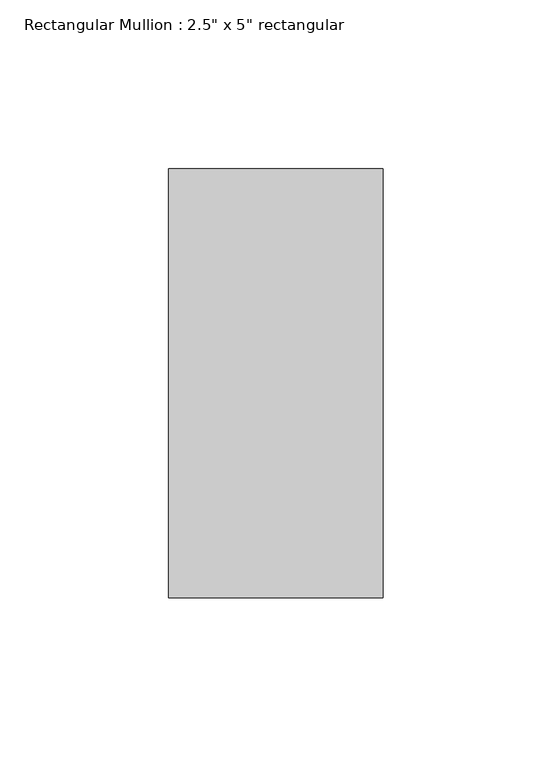
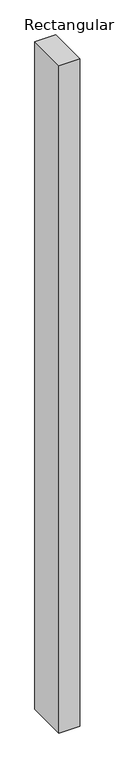
"""IFC4 building model written with IfcOpenShell, lengths in millimetres: member geometry."""

from ifc_helpers import new_model, si_unit, frame, origin, place, context, project, spatial, polyline, outline, extrude, source, transform, mapped, element, save


def member_c08f7e50(model_context):
    return source(origin(), model_context, "Body", "SweptSolid", [
        extrude(outline(polyline([(0.0, 63.5), (0.0, -63.5), (-63.5, -63.5), (-63.5, 63.5), (0.0, 63.5)])), frame((0.0, 0.0, -2159.0), z_axis=(0.0, 0.0, 1.0), x_axis=(1.0, 0.0, 0.0)), (0.0, 0.0, 1.0), 2159.0),
    ])


if __name__ == "__main__":
    model = new_model("IFC4")
    model_context = context("Model", 3, world=origin())
    ifc_project = project(units=[si_unit("LENGTHUNIT", "METRE", prefix="MILLI")], contexts=[model_context])
    site = spatial("IfcSite", under=ifc_project)
    building = spatial("IfcBuilding", under=site)
    placement = place(None, origin())
    member_shape = member_c08f7e50(model_context)
    element("IfcMember", 1, ObjectType="Rectangular Mullion : 2.5\" x 5\" rectangular", at=placement, inside=building, context=model_context, shape_type="MappedRepresentation", body=[
        mapped(member_shape, transform((0.0, 0.0, 0.0), x_axis=(1.0, 0.0, 0.0), y_axis=(0.0, 1.0, 0.0), z_axis=(0.0, 0.0, 1.0))),
    ])
    save(model, "model.ifc")

# Revit data of these elements
# Type "Rectangular Mullion : 2.5\" x 5\" rectangular"
#   built-in parameter 1007304 = 0.416667 (stored number, unit not read)
#   built-in parameter 1007301 = 0.104167 (stored number, unit not read)
#   built-in parameter 1007300 = 0.104167 (stored number, unit not read)
# Element 1 (IfcMember, "Rectangular Mullion : 2.5\" x 5\" rectangular")
#   Materials on its faces: "Aluminum"
# Materials
#   "Aluminum": class "Metal", colour RGB 247 247 247, transparency 0, Description = "Aluminum 6061", Cost = 0
